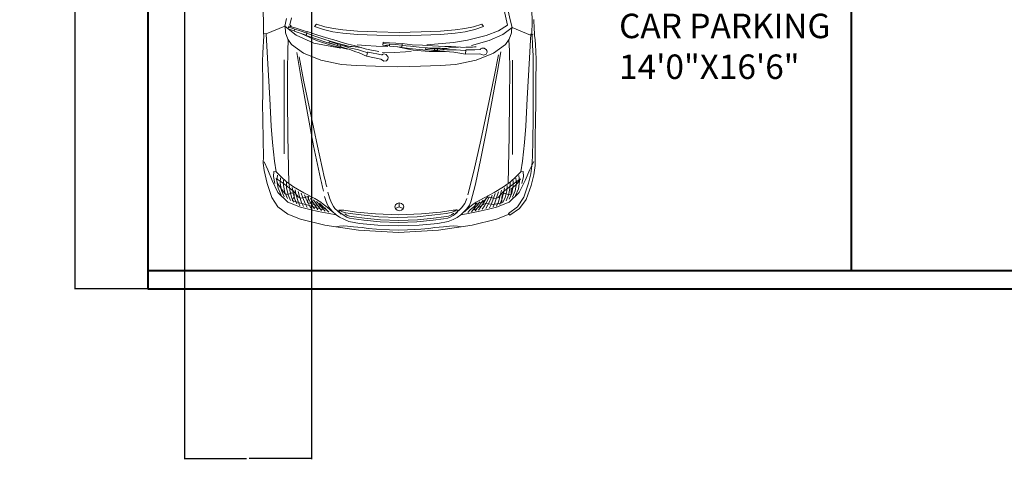
# Model space of a CAD drawing. Units: inches. Extents: x -19 to 419, y -828 to 43.
# Tile 1 of 9: x -9 to 233, y -828 to -720. Entities that reach past the tile are written whole.
import ezdxf

# ---------------------------------------------------------------- set-up
doc = ezdxf.new("R2010")
doc.units = ezdxf.units.IN
doc.header["$MEASUREMENT"] = 0
for name, color, linetype, lineweight in [('A-ANNO-DIMS', 2, 'Continuous', 18), ('A-AREA-IDEN', 7, 'Continuous', 25), ('A-EQPM-VEHI', 8, 'Continuous', 13), ('A-WALL', 7, 'Continuous', 40)]:
    doc.layers.add(name, color=color, linetype=linetype, lineweight=lineweight)
doc.styles.get("Standard").update_dxf_attribs({"font": 'arial.ttf'})
doc.dimstyles.get("Standard").update_dxf_attribs({"dimtxt": 0.18, "dimasz": 0.18, "dimexe": 0.18, "dimexo": 0.0625, "dimgap": 0.09, "dimtad": 0, "dimtih": 1, "dimtoh": 1, "dimdec": 0, "dimzin": 0, "dimdsep": 46, "dimlunit": 3, "dimtxsty": 'Standard', "dimcen": 0.09, "dimadec": 0, "dimazin": 0, "dimtfac": 1, "dimtdec": 0, "dimtofl": 0, "dimtmove": 0, "dimatfit": 3, "dimfxl": 1, "dimtolj": 1, "dimtzin": 0, "dimarcsym": 0})

# ---------------------------------------------------------------- blocks, each defined once
blk = doc.blocks.new('*D2')
at = {"layer": 'A-ANNO-DIMS', "color": 0, "lineweight": -2, "transparency": 16777216}
for p, q in [((22.68, 4.77), (4.74, 4.77)), ((4.92, 4.59), (4.92, -387.33)), ((4.92, -785.55), (4.92, -393.64)), ((22.68, -785.73), (4.74, -785.73))]:
    blk.add_line(p, q, dxfattribs=at)
at = {"layer": 'A-ANNO-DIMS', "color": 0, "transparency": 16777216}
for points in [[(4.89, 4.59), (4.95, 4.59), (4.92, 4.77)], [(4.89, -785.55), (4.95, -785.55), (4.92, -785.73)]]:
    blk.add_solid(points, dxfattribs=at)
at = {"layer": 'Defpoints', "color": 0, "transparency": 16777216}
for p in [(22.74, 4.77), (4.92, -785.73), (22.74, -785.73)]:
    blk.add_point(p, dxfattribs=at)
at = {"layer": 'A-ANNO-DIMS', "color": 0, "transparency": 16777216, "insert": (4.92, -390.48), "char_height": 6, "attachment_point": 5}
blk.add_mtext('\\A1;65\'-11"', dxfattribs=at)
blk = doc.blocks.new('*D49')
at = {"layer": 'A-ANNO-DIMS', "color": 0, "lineweight": -2, "transparency": 16777216}
for p, q in [((31.74, -574.3), (31.74, -827.51)), ((62.91, -574.3), (62.91, -827.51)), ((31.92, -827.33), (46.99, -827.33)), ((62.73, -827.33), (47.65, -827.33))]:
    blk.add_line(p, q, dxfattribs=at)
at = {"layer": 'A-ANNO-DIMS', "color": 0, "transparency": 16777216}
for points in [[(31.92, -827.3), (31.92, -827.36), (31.74, -827.33)], [(62.73, -827.3), (62.73, -827.36), (62.91, -827.33)]]:
    blk.add_solid(points, dxfattribs=at)
at = {"layer": 'Defpoints', "color": 0, "transparency": 16777216}
for p in [(31.74, -574.23), (62.91, -574.23), (62.91, -827.33)]:
    blk.add_point(p, dxfattribs=at)
at = {"layer": 'A-ANNO-DIMS', "color": 0, "transparency": 16777216, "insert": (47.32, -827.33), "char_height": 0.18, "attachment_point": 5}
blk.add_mtext('\\A1;2\'-7"', dxfattribs=at)

msp = doc.modelspace()

# ---------------------------------------------------------------- linework, layer by layer
at = {"layer": 'A-EQPM-VEHI'}
for p, q in [((110.98, -721.14), (106.96, -702.78)), ((51.11, -720.09), (50.99, -716.14)), ((111.66, -719.76), (110.72, -715.68)), ((117, -720.74), (116.97, -716.79)), ((56.35, -721.38), (56.79, -719.49)), ((57.97, -719.3), (57.56, -721.02)), ((51.16, -722.31), (51.11, -720.09)), ((51.81, -723.24), (56.35, -721.38)), ((56.35, -721.38), (59.11, -723.58)), ((56.44, -721.27), (56.56, -723.01)), ((57.2, -721.98), (57.38, -721.33)), ((57.69, -722.17), (57.2, -721.98)), ((58.83, -722.09), (57.31, -721.62)), ((58.88, -721.76), (57.38, -721.33)), ((57.56, -721.02), (57.71, -721.14)), ((57.71, -721.14), (57.86, -721.25)), ((57.86, -721.25), (58.02, -721.35)), ((60.36, -722.23), (58.88, -721.76)), ((64.09, -720.84), (63.65, -721.41)), ((63.65, -721.41), (65.82, -722.13)), ((66.14, -721.49), (64.09, -720.84)), ((68.26, -721.93), (66.14, -721.49)), ((70.58, -722.26), (68.26, -721.93)), ((100.49, -721.93), (98.17, -722.26)), ((102.6, -721.49), (100.49, -721.93)), ((104.65, -720.84), (102.6, -721.49)), ((102.93, -722.13), (105.09, -721.41)), ((105.09, -721.41), (104.65, -720.84)), ((108.74, -722.45), (110.98, -721.14)), ((109.84, -723.36), (112.09, -721.66)), ((112.09, -721.66), (111.66, -719.76)), ((111.95, -723.01), (112.07, -721.27)), ((116.63, -723.51), (112.09, -721.66)), ((116.98, -722.76), (117, -720.74)), ((117.4, -719.74), (117.5, -721.96)), ((117.5, -721.96), (117.56, -723.07)), ((51.15, -725.07), (51.2, -723.75)), ((51.17, -723.01), (51.16, -722.31)), ((51.2, -723.75), (51.17, -723.01)), ((51.18, -723.05), (51.81, -723.24)), ((52.13, -729.21), (51.82, -723.2)), ((56.56, -723.01), (57.09, -724.56)), ((58.19, -722.35), (57.69, -722.17)), ((58.68, -722.52), (58.19, -722.35)), ((58.68, -722.52), (58.83, -722.09)), ((59.65, -722.89), (58.68, -722.56)), ((60.15, -722.5), (58.83, -722.09)), ((59.11, -723.58), (63.48, -725.48)), ((60.63, -723.2), (59.65, -722.89)), ((60.15, -722.5), (61.74, -723.08)), ((61.83, -722.74), (60.36, -722.23)), ((60.55, -723.19), (64.14, -724.83)), ((61.6, -723.53), (60.63, -723.2)), ((61.58, -723.61), (61.83, -722.74)), ((64.01, -724.46), (61.58, -723.61)), ((61.72, -723.1), (63.71, -723.78)), ((64.18, -723.49), (61.85, -722.67)), ((63.71, -723.78), (65.69, -724.46)), ((66.46, -725.3), (64.01, -724.46)), ((66.58, -724.21), (64.18, -723.49)), ((65.69, -724.46), (67.69, -725.11)), ((65.82, -722.13), (68.14, -722.7)), ((68.96, -724.89), (66.58, -724.21)), ((68.14, -722.7), (70.58, -723.1)), ((74.17, -722.54), (70.58, -722.26)), ((70.58, -723.1), (74.17, -723.38)), ((78.91, -722.73), (74.17, -722.54)), ((74.17, -723.38), (78.91, -723.57)), ((84.37, -722.87), (78.91, -722.73)), ((78.91, -723.57), (84.37, -723.71)), ((89.83, -722.73), (84.37, -722.87)), ((84.37, -723.71), (89.83, -723.57)), ((94.58, -722.54), (89.83, -722.73)), ((89.83, -723.57), (94.58, -723.38)), ((98.17, -722.26), (94.58, -722.54)), ((94.58, -723.38), (98.17, -723.1)), ((98.17, -723.1), (100.61, -722.7)), ((100.61, -722.7), (102.93, -722.13)), ((102.13, -724.57), (105.78, -723.61)), ((105.78, -723.61), (108.74, -722.45)), ((106.51, -724.84), (109.84, -723.36)), ((111.42, -724.56), (111.95, -723.01)), ((116.37, -729.21), (116.69, -723.2)), ((117.27, -723.32), (116.63, -723.51)), ((116.97, -723.32), (116.98, -722.76)), ((116.97, -723.39), (116.97, -723.32)), ((116.99, -723.45), (116.97, -723.39)), ((117.01, -723.5), (116.99, -723.45)), ((117.12, -726.05), (117.01, -723.5)), ((117.56, -723.07), (117.61, -723.63)), ((117.61, -723.63), (117.73, -724.68)), ((50.94, -728), (51.04, -726.41)), ((51.04, -726.41), (51.15, -725.07)), ((57.06, -727.37), (57.21, -724.68)), ((57.09, -724.56), (57.98, -725.84)), ((57.98, -725.84), (60.96, -727.96)), ((63.48, -725.48), (70.08, -726.76)), ((64.14, -724.83), (67.9, -726.05)), ((68.94, -725.99), (66.46, -725.3)), ((67.15, -725.34), (67.28, -725.04)), ((67.15, -725.34), (68.06, -725.7)), ((68.17, -725.38), (67.26, -725.04)), ((67.69, -725.11), (69.23, -725.52)), ((67.9, -726.05), (71.74, -726.97)), ((68.06, -725.7), (68.99, -726.04)), ((69.11, -725.71), (68.17, -725.38)), ((70.43, -725.32), (68.96, -724.89)), ((68.99, -726.04), (69.93, -726.32)), ((70.04, -725.99), (69.11, -725.71)), ((69.21, -726.1), (69.32, -725.78)), ((69.23, -725.52), (70.77, -725.9)), ((69.92, -726.3), (70.04, -725.92)), ((69.92, -726.34), (70.42, -726.5)), ((70.04, -725.92), (71.22, -726.33)), ((70.42, -726.5), (70.94, -726.67)), ((71.9, -725.75), (70.43, -725.32)), ((70.77, -725.9), (72.3, -726.3)), ((70.94, -726.67), (71.45, -726.83)), ((71, -726.17), (71.63, -726.27)), ((71.22, -726.33), (72.16, -726.63)), ((71.45, -726.83), (72.58, -727.18)), ((71.63, -726.27), (72.27, -726.29)), ((73.39, -726.1), (71.9, -725.75)), ((72.16, -726.63), (73.34, -726.9)), ((72.27, -726.29), (72.9, -726.32)), ((75.11, -726.61), (72.9, -726.32)), ((76.68, -727.06), (73.39, -726.1)), ((74.07, -725.9), (76.23, -726.11)), ((76.23, -726.11), (78.77, -726.26)), ((78.77, -726.26), (81.66, -726.31)), ((80.44, -725.98), (80.47, -725.3)), ((80.96, -726.05), (80.44, -725.98)), ((82.03, -725.39), (80.47, -725.3)), ((82.05, -725.72), (80.47, -725.6)), ((81.49, -726.12), (80.96, -726.05)), ((82.01, -726.17), (81.49, -726.12)), ((82.01, -726.17), (82.05, -725.72)), ((83.04, -726.31), (82.02, -726.21)), ((83.58, -725.51), (82.03, -725.39)), ((83.43, -725.82), (82.05, -725.72)), ((84.06, -726.4), (83.04, -726.31)), ((83.43, -725.82), (85.11, -726.03)), ((85.13, -725.68), (83.58, -725.51)), ((83.98, -726.4), (87.85, -727.19)), ((85.08, -726.5), (84.06, -726.4)), ((85.07, -726.58), (85.13, -725.68)), ((87.64, -726.86), (85.07, -726.58)), ((85.1, -726.05), (87.19, -726.26)), ((87.58, -725.88), (85.13, -725.6)), ((87.19, -726.26), (89.28, -726.49)), ((90.09, -726.04), (87.58, -725.88)), ((90.21, -727.13), (87.64, -726.86)), ((89.28, -726.49), (91.37, -726.67)), ((92.55, -726.17), (90.09, -726.04)), ((90.89, -727.02), (90.95, -726.69)), ((91.9, -726.82), (90.93, -726.69)), ((91.22, -725.93), (97.71, -725.34)), ((91.37, -726.67), (92.96, -726.73)), ((92.88, -726.94), (91.9, -726.82)), ((94.08, -726.26), (92.55, -726.17)), ((92.96, -726.73), (94.54, -726.75)), ((95.62, -726.34), (94.08, -726.26)), ((94.54, -726.75), (96.13, -726.79)), ((95.47, -726.92), (96.09, -726.79)), ((97.14, -726.35), (95.62, -726.34)), ((96.09, -726.79), (96.72, -726.67)), ((98.93, -726.46), (96.72, -726.67)), ((100.57, -726.55), (97.14, -726.35)), ((97.71, -725.34), (101.13, -724.8)), ((101.13, -726.51), (100.73, -726.53)), ((101.13, -724.8), (102.13, -724.57)), ((101.54, -726.5), (101.13, -726.51)), ((101.94, -726.49), (101.54, -726.5)), ((102.4, -726.46), (101.94, -726.49)), ((102.13, -726.05), (106.51, -724.84)), ((102.87, -726.44), (102.4, -726.46)), ((103.33, -726.45), (102.87, -726.44)), ((104.39, -726.91), (104.71, -726.72)), ((104.71, -726.72), (105.23, -726.72)), ((105.23, -726.72), (105.59, -726.95)), ((107.55, -727.96), (110.52, -725.84)), ((110.52, -725.84), (111.42, -724.56)), ((111.45, -727.37), (111.29, -724.68)), ((117.31, -728.53), (117.12, -726.05)), ((117.73, -724.68), (117.86, -725.89)), ((117.86, -725.89), (117.96, -727.53)), ((50.89, -729.91), (50.94, -728)), ((52.68, -739.06), (52.13, -729.21)), ((56.99, -732.11), (57.06, -727.37)), ((60.27, -733.68), (59.27, -727.8)), ((60.97, -734.55), (59.89, -728.86)), ((60.96, -727.96), (65.23, -729.67)), ((72.58, -727.18), (73.53, -727.55)), ((73.34, -726.9), (74.42, -727.16)), ((73.53, -727.55), (74.63, -727.92)), ((74.42, -727.16), (75.45, -727.47)), ((74.63, -727.92), (75.18, -728.15)), ((75.18, -728.15), (75.85, -728.47)), ((75.45, -727.47), (76.51, -727.79)), ((75.85, -728.47), (76.39, -728.72)), ((76.39, -728.72), (76.71, -727.65)), ((79.87, -729.45), (76.41, -728.67)), ((76.81, -727.71), (78.01, -727.97)), ((77.59, -727.21), (76.84, -727.08)), ((78.63, -727.41), (77.59, -727.21)), ((78.01, -727.97), (78.9, -728.16)), ((79.39, -727.59), (78.63, -727.41)), ((78.9, -728.16), (80.11, -728.41)), ((80.21, -727.89), (83.3, -727.79)), ((80.21, -728.44), (80.27, -728.39)), ((80.27, -728.39), (80.32, -728.28)), ((80.32, -728.28), (80.68, -728.16)), ((80.68, -728.16), (81.18, -728.27)), ((81.18, -728.27), (81.49, -728.58)), ((81.49, -728.58), (81.59, -728.76)), ((81.59, -728.76), (81.67, -729.03)), ((81.67, -729.03), (81.66, -729.44)), ((83.3, -727.79), (85.97, -727.64)), ((85.97, -727.64), (87.39, -727.57)), ((87.85, -727.19), (91.78, -727.54)), ((92.78, -727.25), (90.21, -727.13)), ((90.89, -727.02), (91.86, -727.16)), ((91.78, -727.54), (95.73, -727.57)), ((91.86, -727.16), (92.85, -727.28)), ((92.85, -727.28), (93.83, -727.34)), ((93.86, -727), (92.88, -726.94)), ((93.07, -727.29), (93.1, -726.95)), ((93.8, -727.33), (93.84, -726.93)), ((93.81, -727.36), (94.34, -727.4)), ((93.84, -726.93), (95.08, -727.06)), ((94.34, -727.4), (94.89, -727.45)), ((94.83, -726.96), (95.47, -726.92)), ((94.89, -727.45), (95.42, -727.49)), ((95.08, -727.06), (96.06, -727.15)), ((95.42, -727.49), (96.75, -727.61)), ((96.06, -727.15), (97.28, -727.14)), ((96.75, -727.61), (97.83, -727.75)), ((97.28, -727.14), (98.39, -727.16)), ((97.83, -727.75), (99.26, -727.94)), ((98.39, -727.16), (99.46, -727.23)), ((99.26, -727.94), (99.72, -728.03)), ((99.46, -727.23), (100.56, -727.3)), ((99.72, -728.03), (100.2, -728.14)), ((100.2, -728.14), (100.66, -728.23)), ((100.66, -728.23), (100.72, -727.11)), ((104.21, -728.16), (100.66, -728.18)), ((100.84, -727.15), (102.06, -727.13)), ((102.06, -727.13), (102.98, -727.12)), ((102.98, -727.12), (104.21, -727.09)), ((103.28, -729.67), (107.55, -727.96)), ((104.7, -728.29), (104.21, -728.16)), ((104.31, -727.09), (104.36, -727.03)), ((104.36, -727.03), (104.39, -726.91)), ((105.11, -728.45), (104.7, -728.29)), ((105.73, -728.24), (105.11, -728.45)), ((105.59, -726.95), (105.73, -727.1)), ((105.73, -727.1), (105.87, -727.34)), ((105.96, -727.74), (105.73, -728.24)), ((105.87, -727.34), (105.96, -727.74)), ((107.68, -733.79), (108.76, -728.36)), ((108.51, -732.41), (109.33, -727.6)), ((111.52, -732.11), (111.45, -727.37)), ((115.83, -739.06), (116.37, -729.21)), ((117.31, -731.08), (117.31, -728.53)), ((117.96, -727.53), (118.01, -729.53)), ((50.92, -731.36), (50.89, -729.91)), ((50.95, -733.97), (50.92, -731.36)), ((56.16, -729.6), (56.16, -752.6)), ((65.23, -729.67), (70.28, -730.72)), ((70.28, -730.72), (73.87, -731)), ((73.87, -731), (78.62, -731.19)), ((78.62, -731.19), (84.08, -731.33)), ((80.32, -729.69), (79.87, -729.45)), ((80.68, -729.94), (80.32, -729.69)), ((81.33, -729.87), (80.68, -729.94)), ((81.66, -729.44), (81.33, -729.87)), ((84.08, -731.33), (89.63, -731.19)), ((89.63, -731.19), (94.54, -731)), ((94.54, -731), (98.22, -730.72)), ((98.22, -730.72), (103.28, -729.67)), ((112.18, -729.67), (112.18, -752.77)), ((117.27, -733.77), (117.31, -731.08)), ((117.99, -731.04), (117.93, -733.74)), ((118.01, -729.53), (117.99, -731.04)), ((50.93, -738.02), (50.95, -733.97)), ((57.01, -739.03), (56.99, -732.11)), ((61.74, -741.8), (60.27, -733.68)), ((106.17, -741.19), (107.68, -733.79)), ((107.32, -739), (108.51, -732.41)), ((111.5, -739.03), (111.52, -732.11)), ((117.27, -737.94), (117.27, -733.77)), ((117.93, -733.74), (117.9, -737.93)), ((62.54, -742.29), (60.97, -734.55)), ((50.92, -740.67), (50.93, -738.02)), ((117.27, -740.67), (117.27, -737.94)), ((117.9, -737.93), (117.89, -740.67)), ((50.98, -743.95), (50.92, -740.67)), ((53.04, -745.88), (52.68, -739.06)), ((57.12, -748.25), (57.01, -739.03)), ((104.44, -749.31), (106.17, -741.19)), ((105.91, -746.44), (107.32, -739)), ((111.38, -748.25), (111.5, -739.03)), ((115.47, -745.88), (115.83, -739.06)), ((117.25, -743.95), (117.27, -740.67)), ((117.89, -740.67), (117.84, -743.87)), ((63.43, -750.66), (61.74, -741.8)), ((64.34, -750.75), (62.54, -742.29)), ((51.09, -749.34), (50.98, -743.95)), ((53.35, -749.9), (53.04, -745.88)), ((115.15, -749.9), (115.47, -745.88)), ((117.2, -749.35), (117.25, -743.95)), ((117.84, -743.87), (117.76, -749.11)), ((57.34, -759.88), (57.12, -748.25)), ((104.45, -753.79), (105.91, -746.44)), ((111.17, -759.88), (111.38, -748.25)), ((51.11, -753.26), (51.09, -749.34)), ((53.85, -754.4), (53.35, -749.9)), ((65.1, -758.72), (63.43, -750.66)), ((66.13, -758.62), (64.34, -750.75)), ((102.73, -756.89), (104.44, -749.31)), ((114.65, -754.4), (115.15, -749.9)), ((117.1, -753.27), (117.2, -749.35)), ((117.76, -749.11), (117.76, -752.94)), ((51.07, -754.93), (51.11, -753.26)), ((116.95, -755.57), (117.1, -753.27)), ((117.76, -752.94), (117.73, -755.49)), ((51.29, -756.75), (51.07, -754.93)), ((52.19, -756.52), (51.28, -754.59)), ((54.26, -757.05), (53.85, -754.4)), ((103.09, -760.09), (104.45, -753.79)), ((114.25, -757.05), (114.65, -754.4)), ((117.4, -754.48), (116.44, -756.44)), ((116.69, -757.5), (116.95, -755.57)), ((117.73, -755.49), (117.43, -757.82)), ((52.07, -759.88), (51.29, -756.75)), ((53.26, -759.17), (52.19, -756.52)), ((53.62, -758.16), (53.68, -756.99)), ((53.95, -759.87), (53.62, -758.16)), ((53.68, -756.99), (54.26, -757.05)), ((54.26, -757.05), (55.44, -758.29)), ((54.43, -759.26), (54.6, -757.89)), ((55.44, -758.29), (56.75, -759.48)), ((101.25, -762.66), (102.73, -756.89)), ((113.06, -758.29), (111.75, -759.48)), ((114.25, -757.05), (113.06, -758.29)), ((113.95, -759.35), (113.78, -757.99)), ((114.83, -757), (114.25, -757.05)), ((114.53, -759.93), (114.88, -758.2)), ((114.88, -758.2), (114.83, -757)), ((116.44, -756.44), (115.29, -759.15)), ((116.15, -759.8), (116.69, -757.5)), ((117.43, -757.82), (116.82, -760.36)), ((53.21, -763.32), (52.07, -759.88)), ((54.64, -762.13), (53.26, -759.17)), ((55.71, -759.7), (54.24, -758.67)), ((54.24, -758.67), (54.67, -760.02)), ((54.73, -761.08), (54.43, -759.26)), ((54.67, -760.02), (55.83, -761.65)), ((55.22, -759.84), (55.32, -758.49)), ((55.55, -761.61), (55.22, -759.84)), ((58.39, -761.74), (55.71, -759.7)), ((56.01, -760.42), (56.03, -759.08)), ((56.36, -762.15), (56.01, -760.42)), ((56.75, -759.48), (58.5, -760.71)), ((56.8, -761), (56.75, -759.67)), ((57.59, -761.58), (57.46, -760.27)), ((65.32, -759.68), (65.1, -758.72)), ((65.6, -760.84), (65.32, -759.68)), ((66.3, -759.32), (66.13, -758.62)), ((66.46, -760.03), (66.3, -759.32)), ((66.63, -760.74), (66.46, -760.03)), ((102, -764.42), (103.09, -760.09)), ((109.98, -761.84), (112.67, -759.8)), ((111.75, -759.48), (110.01, -760.71)), ((110.79, -761.68), (110.91, -760.37)), ((111.58, -761.1), (111.63, -759.77)), ((113.36, -759.89), (111.85, -761.28)), ((112.01, -762.25), (112.37, -760.52)), ((112.37, -760.52), (112.34, -759.18)), ((112.67, -759.8), (114.14, -758.77)), ((112.83, -761.71), (113.16, -759.93)), ((113.16, -759.93), (113.06, -758.59)), ((114.14, -758.77), (113.36, -759.89)), ((113.64, -761.18), (113.95, -759.35)), ((115.29, -759.15), (113.86, -762.13)), ((114.95, -763.27), (116.15, -759.8)), ((116.82, -760.36), (115.57, -763.8)), ((57.1, -764.45), (54.64, -762.13)), ((55.43, -762.75), (54.73, -761.08)), ((56.21, -763.19), (55.55, -761.61)), ((55.83, -761.65), (56.48, -762.44)), ((56.98, -763.62), (56.36, -762.15)), ((56.48, -762.44), (57.1, -762.6)), ((57.18, -762.68), (56.8, -761)), ((57.1, -762.6), (58.05, -762.22)), ((57.75, -764.06), (57.18, -762.68)), ((57.99, -763.22), (57.59, -761.58)), ((58.05, -762.22), (58.66, -762.53)), ((58.38, -762.16), (58.18, -760.86)), ((58.8, -763.75), (58.38, -762.16)), ((59.73, -763.23), (58.39, -761.74)), ((58.5, -760.71), (61.06, -762.17)), ((58.66, -762.53), (58.63, -763.16)), ((59.17, -762.74), (58.9, -761.46)), ((59.62, -764.29), (59.17, -762.74)), ((59.98, -763.09), (59.65, -761.86)), ((60.48, -764.54), (59.98, -763.09)), ((60.8, -763.44), (60.4, -762.27)), ((61.06, -762.17), (63.73, -763.61)), ((61.61, -763.78), (61.15, -762.68)), ((62.23, -763.05), (61.54, -763.25)), ((62.42, -764.13), (61.9, -763.09)), ((61.94, -764.56), (62.23, -763.05)), ((65.83, -761.8), (65.6, -760.84)), ((66.41, -764.07), (66.1, -763.1)), ((67.32, -763.42), (66.91, -762.05)), ((107.71, -762.08), (105.29, -763.42)), ((106.77, -763.88), (107.23, -762.78)), ((107.58, -763.53), (107.98, -762.37)), ((110.01, -760.71), (107.71, -762.08)), ((108.39, -763.19), (108.73, -761.96)), ((108.65, -763.33), (109.98, -761.84)), ((108.76, -764.39), (109.21, -762.84)), ((109.21, -762.84), (109.48, -761.56)), ((109.57, -763.85), (110, -762.26)), ((109.72, -762.63), (109.58, -763.38)), ((110.32, -762.32), (109.72, -762.63)), ((110, -762.26), (110.2, -760.96)), ((111.28, -762.69), (110.32, -762.32)), ((110.39, -763.32), (110.79, -761.68)), ((110.63, -764.16), (111.2, -762.78)), ((111.2, -762.78), (111.58, -761.1)), ((111.89, -762.54), (111.28, -762.69)), ((113.86, -762.13), (111.4, -764.45)), ((111.4, -763.72), (112.01, -762.25)), ((111.85, -761.28), (111.89, -762.54)), ((112.17, -763.29), (112.83, -761.71)), ((112.95, -762.85), (113.64, -761.18)), ((54.68, -765.67), (53.21, -763.32)), ((60.23, -765.73), (57.1, -764.45)), ((58.52, -764.5), (57.99, -763.22)), ((58.32, -763.77), (58.13, -764.04)), ((58.13, -764.04), (60.24, -764.76)), ((58.63, -763.16), (58.32, -763.77)), ((59.3, -764.93), (58.8, -763.75)), ((60.07, -765.37), (59.62, -764.29)), ((60.29, -763.49), (59.73, -763.23)), ((60.24, -764.76), (61.74, -765.18)), ((61.54, -763.25), (60.29, -763.49)), ((60.95, -765.56), (60.48, -764.54)), ((61.34, -764.79), (60.8, -763.44)), ((61.83, -765.76), (61.34, -764.79)), ((62.21, -765.03), (61.61, -763.78)), ((61.74, -765.18), (62.32, -765.32)), ((66.38, -765.93), (61.94, -764.56)), ((62.72, -765.95), (62.21, -765.03)), ((62.32, -765.32), (65.6, -766.28)), ((63.07, -765.28), (62.42, -764.13)), ((63.23, -764.48), (62.65, -763.5)), ((63.6, -766.15), (63.07, -765.28)), ((63.93, -765.53), (63.23, -764.48)), ((64.04, -764.83), (63.4, -763.91)), ((63.73, -763.61), (65.18, -764.5)), ((64.48, -766.34), (63.93, -765.53)), ((64.79, -765.78), (64.04, -764.83)), ((64.86, -765.18), (64.15, -764.31)), ((65.65, -766.03), (64.86, -765.18)), ((65.67, -765.53), (64.9, -764.72)), ((65.18, -764.5), (65.78, -764.99)), ((66.52, -766.27), (65.67, -765.53)), ((65.78, -764.99), (66.77, -765.71)), ((66.76, -764.95), (66.41, -764.07)), ((67.17, -765.72), (66.76, -764.95)), ((67.83, -764.66), (67.32, -763.42)), ((68.32, -765.58), (67.83, -764.66)), ((83.36, -765.61), (83.5, -765.13)), ((83.5, -765.13), (83.89, -764.79)), ((83.89, -764.79), (84.44, -764.66)), ((84.44, -764.66), (84.99, -764.79)), ((84.44, -765.61), (84.44, -764.66)), ((84.99, -764.79), (85.38, -765.13)), ((85.38, -765.13), (85.52, -765.61)), ((99.69, -765.89), (100.48, -764.82)), ((100.48, -764.82), (100.84, -763.98)), ((100.84, -763.98), (100.97, -763.58)), ((100.96, -766.23), (101.68, -765.23)), ((102.55, -764.98), (101.65, -765.7)), ((101.68, -765.23), (102, -764.42)), ((103.33, -764.5), (102.55, -764.98)), ((102.71, -765.63), (103.48, -764.82)), ((102.72, -766.12), (103.52, -765.28)), ((105.65, -764.71), (102.78, -766.38)), ((102.78, -766.38), (103.13, -764.85)), ((103.13, -764.85), (104.96, -764.51)), ((105.29, -763.42), (103.33, -764.5)), ((103.52, -765.28), (104.23, -764.41)), ((103.59, -765.88), (104.33, -764.93)), ((104.33, -764.93), (104.98, -764)), ((104.45, -765.63), (105.15, -764.58)), ((104.78, -766.24), (105.31, -765.38)), ((104.96, -764.51), (106.15, -763.15)), ((105.15, -764.58), (105.73, -763.6)), ((105.31, -765.38), (105.96, -764.23)), ((106.17, -764.87), (105.65, -764.71)), ((105.66, -766.05), (106.17, -765.13)), ((105.96, -764.23), (106.48, -763.19)), ((106.15, -763.15), (106.84, -763.35)), ((106.17, -765.13), (106.77, -763.88)), ((107.57, -765.02), (106.17, -764.87)), ((106.54, -765.86), (107.03, -764.88)), ((106.84, -763.35), (108.09, -763.59)), ((107.03, -764.88), (107.58, -763.53)), ((107.43, -765.66), (107.9, -764.64)), ((109.61, -764.61), (107.57, -765.02)), ((107.9, -764.64), (108.39, -763.19)), ((108.09, -763.59), (108.65, -763.33)), ((111.4, -764.45), (108.27, -765.73)), ((108.31, -765.47), (108.76, -764.39)), ((109.08, -765.03), (109.57, -763.85)), ((109.58, -763.38), (109.59, -764.21)), ((109.59, -764.21), (109.61, -764.61)), ((109.85, -764.59), (110.39, -763.32)), ((113.43, -765.62), (114.95, -763.27)), ((115.57, -763.8), (113.93, -766.07)), ((57.08, -767.46), (54.68, -765.67)), ((60.22, -768.66), (57.08, -767.46)), ((62.48, -766.3), (60.23, -765.73)), ((64.55, -766.75), (62.48, -766.3)), ((67.21, -767.28), (64.55, -766.75)), ((65.37, -766.54), (64.79, -765.78)), ((65.6, -766.28), (66.38, -765.93)), ((66.25, -766.73), (65.65, -766.03)), ((67.13, -766.92), (66.52, -766.27)), ((66.77, -765.71), (68.07, -766.88)), ((67.49, -766.16), (67.17, -765.72)), ((68.97, -767.59), (67.21, -767.28)), ((68.09, -766.76), (67.49, -766.16)), ((68.97, -767.59), (68.09, -766.76)), ((68.65, -766.01), (68.32, -765.58)), ((69.26, -766.6), (68.65, -766.01)), ((69.79, -768.14), (68.97, -767.59)), ((70.15, -767.41), (69.26, -766.6)), ((69.63, -766.44), (70.83, -766.43)), ((69.86, -767), (69.63, -766.44)), ((70.89, -767.78), (69.86, -767)), ((70.53, -766.84), (69.88, -766.5)), ((71.31, -767.06), (70.53, -766.84)), ((70.83, -766.43), (73.92, -766.9)), ((71.57, -768.2), (70.89, -767.78)), ((71.54, -767.68), (71.04, -767.31)), ((72.4, -767.24), (71.31, -767.06)), ((72.23, -767.93), (71.54, -767.68)), ((73.37, -768.12), (72.23, -767.93)), ((75.09, -767.59), (72.4, -767.24)), ((73.92, -766.9), (78.59, -767.37)), ((79.4, -768.05), (75.09, -767.59)), ((78.59, -767.37), (84.32, -767.59)), ((83.5, -766.1), (83.36, -765.61)), ((83.47, -766.03), (84.44, -765.61)), ((83.89, -766.44), (83.5, -766.1)), ((84.44, -766.57), (83.89, -766.44)), ((84.32, -767.59), (89.9, -767.37)), ((84.44, -765.61), (85.41, -766.03)), ((84.99, -766.44), (84.44, -766.57)), ((85.38, -766.1), (84.99, -766.44)), ((85.52, -765.61), (85.38, -766.1)), ((93.18, -767.59), (88.83, -768.05)), ((89.9, -767.37), (94.57, -766.9)), ((95.9, -767.24), (93.18, -767.59)), ((94.57, -766.9), (97.68, -766.43)), ((96.51, -767.92), (95.34, -768.12)), ((97.17, -767.01), (95.9, -767.24)), ((97.24, -767.63), (96.51, -767.92)), ((97.61, -767.78), (96.93, -768.2)), ((98.02, -766.69), (97.17, -767.01)), ((97.78, -767.17), (97.24, -767.63)), ((98.64, -767), (97.61, -767.78)), ((97.68, -766.43), (98.87, -766.44)), ((98.47, -766.28), (98.02, -766.69)), ((98.2, -767.25), (99.69, -765.89)), ((98.87, -766.44), (98.64, -767)), ((99.54, -767.59), (98.65, -768.23)), ((99.54, -767.59), (100.96, -766.23)), ((100.94, -767.32), (99.54, -767.59)), ((101.65, -765.7), (100.44, -766.88)), ((103.77, -766.78), (100.94, -767.32)), ((101.25, -767.02), (101.86, -766.37)), ((101.86, -766.37), (102.71, -765.63)), ((102.13, -766.83), (102.72, -766.12)), ((103.01, -766.63), (103.59, -765.88)), ((106.03, -766.3), (103.77, -766.78)), ((103.89, -766.44), (104.45, -765.63)), ((108.27, -765.73), (106.03, -766.3)), ((108.29, -768.66), (111.42, -767.46)), ((111.25, -767.23), (113.43, -765.62)), ((111.56, -767.69), (111.25, -767.23)), ((113.93, -766.07), (111.56, -767.69)), ((66.21, -770.12), (60.22, -768.66)), ((74.43, -771.37), (66.21, -770.12)), ((68.9, -770.54), (69.78, -770.36)), ((69.78, -770.36), (70.81, -770.31)), ((70.85, -768.67), (69.79, -768.14)), ((70.81, -770.31), (71.73, -770.35)), ((72.05, -769.19), (70.85, -768.67)), ((72.19, -768.44), (71.57, -768.2)), ((71.73, -770.35), (73.23, -770.5)), ((74.66, -769.7), (72.05, -769.19)), ((73.27, -768.61), (72.19, -768.44)), ((75.77, -768.93), (73.27, -768.61)), ((75.87, -768.44), (73.37, -768.12)), ((79.16, -770.11), (74.66, -769.7)), ((79.74, -769.32), (75.77, -768.93)), ((79.83, -768.83), (75.87, -768.44)), ((84.25, -770.28), (79.16, -770.11)), ((84.1, -768.28), (79.4, -768.05)), ((84.25, -769.51), (79.74, -769.32)), ((84.35, -769.02), (79.83, -768.83)), ((88.83, -768.05), (84.1, -768.28)), ((88.77, -769.32), (84.25, -769.51)), ((89.34, -770.11), (84.25, -770.28)), ((88.87, -768.83), (84.35, -769.02)), ((92.73, -768.93), (88.77, -769.32)), ((92.83, -768.44), (88.87, -768.83)), ((93.85, -769.7), (89.34, -770.11)), ((95.24, -768.61), (92.73, -768.93)), ((95.34, -768.12), (92.83, -768.44)), ((96.46, -769.19), (93.85, -769.7)), ((94.07, -771.37), (102.29, -770.12)), ((96.31, -768.44), (95.24, -768.61)), ((96.78, -770.35), (95.28, -770.5)), ((96.93, -768.2), (96.31, -768.44)), ((97.62, -768.72), (96.46, -769.19)), ((97.7, -770.31), (96.78, -770.35)), ((98.65, -768.23), (97.62, -768.72)), ((98.73, -770.36), (97.7, -770.31)), ((99.6, -770.54), (98.73, -770.36)), ((102.29, -770.12), (108.29, -768.66)), ((73.23, -770.5), (75.34, -770.73)), ((84.25, -771.95), (74.43, -771.37)), ((75.34, -770.73), (76.8, -770.93)), ((76.8, -770.93), (78.82, -771.08)), ((78.82, -771.08), (82.02, -771.24)), ((82.02, -771.24), (84.25, -771.31)), ((86.48, -771.24), (84.25, -771.31)), ((84.25, -771.95), (94.07, -771.37)), ((89.69, -771.08), (86.48, -771.24)), ((91.7, -770.93), (89.69, -771.08)), ((93.16, -770.73), (91.7, -770.93)), ((95.28, -770.5), (93.16, -770.73))]:
    msp.add_line(p, q, dxfattribs=at)
at = {"layer": 'A-WALL'}
for p, q in [((22.74, 4.77), (22.74, -785.73)), ((195.24, -583.23), (195.24, -781.23)), ((22.74, -781.23), (409.74, -781.23)), ((22.74, -785.73), (409.74, -785.73))]:
    msp.add_line(p, q, dxfattribs=at)

# ---------------------------------------------------------------- texts
at = {"layer": 'A-AREA-IDEN', "insert": (138.35, -718.29), "char_height": 6, "attachment_point": 1}
msp.add_mtext('CAR PARKING\\P14\'0"X16\'6"', dxfattribs=at)

# ---------------------------------------------------------------- dimensions: what is measured, and where the dimension line sits
at = {"layer": 'A-ANNO-DIMS'}
dim = msp.add_linear_dim(base=(4.917623, -785.73343372), p1=(22.73889525, 4.76656628), p2=(22.73889525, -785.73343372), angle=90, dimstyle='Standard', override={"dimtxt": 6, "dimclrd": 0, "dimclre": 0, "dimclrt": 0}, dxfattribs=at)
dim.commit()
dim.dimension.update_dxf_attribs({"geometry": '*D2', "text_midpoint": (4.917623, -390.48343372)})
dim = msp.add_linear_dim(base=(62.91, -827.33), p1=(31.74, -574.23), p2=(62.91, -574.23), dimstyle='Standard', override={"dimdec": 1, "dimlfac": 1, "dimrnd": 0, "dimzin": 1, "dimdsep": 46, "dimlunit": 4, "dimfrac": 2}, dxfattribs=at)
dim.commit()
dim.dimension.update_dxf_attribs({"geometry": '*D49', "text_midpoint": (47.32, -827.33)})

doc.saveas('drawing.dxf')
